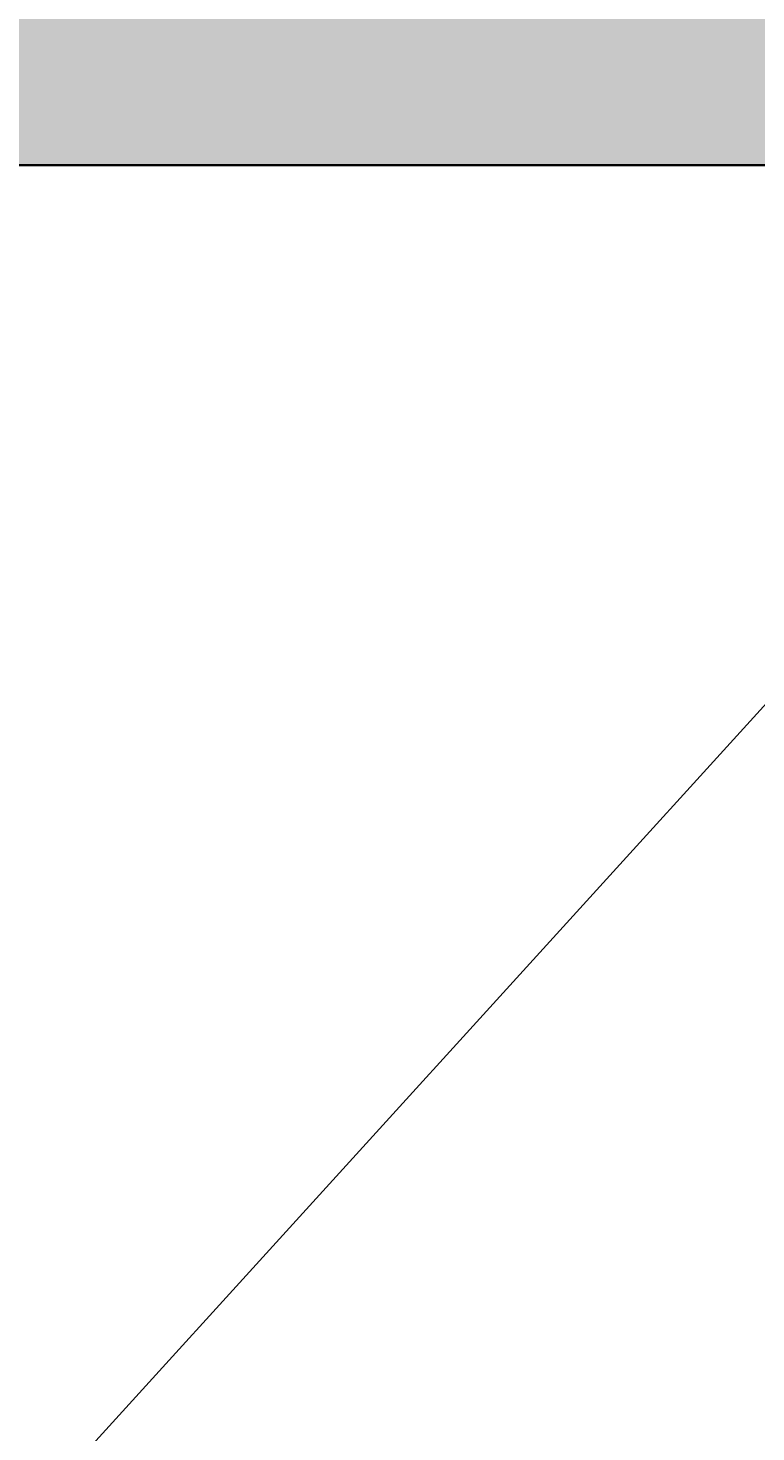
# Model space of a CAD drawing. Units: inches. Extents: x 1998 to 2588, y 1139 to 1977.
# Tile 37 of 134: x 2257 to 2275, y 1557 to 1592. Entities that reach past the tile are written whole.
import ezdxf

# ---------------------------------------------------------------- set-up
doc = ezdxf.new("R2010")
doc.units = ezdxf.units.IN
for name, color, linetype, lineweight in [('A-ANNO-DIMS', 2, 'Continuous', 18), ('A-FLOR-OPEN', 8, 'Continuous', 18), ('A-WALL-PATT', 252, 'Continuous', 13), ('WALL', 200, 'Continuous', 35)]:
    doc.layers.add(name, color=color, linetype=linetype, lineweight=lineweight)
doc.styles.get("Standard").update_dxf_attribs({"font": 'arial.ttf'})
doc.dimstyles.get("Standard").update_dxf_attribs({"dimtxt": 0.18, "dimasz": 0.18, "dimexe": 0.18, "dimexo": 0.0625, "dimgap": 0.09, "dimtad": 0, "dimtih": 1, "dimtoh": 1, "dimdec": 4, "dimzin": 0, "dimdsep": 46, "dimtxsty": 'Standard', "dimcen": 0.09, "dimadec": 0, "dimazin": 0, "dimtfac": 1, "dimtdec": 4, "dimtofl": 0, "dimtmove": 0, "dimatfit": 3, "dimfxl": 1, "dimtolj": 1, "dimtzin": 0, "dimarcsym": 0})

# ---------------------------------------------------------------- blocks, each defined once
blk = doc.blocks.new('*D34')
at = {"layer": 'A-ANNO-DIMS', "color": 0, "lineweight": -2, "transparency": 16777216}
for p, q in [((2407.91, 1594.732), (1997.843, 1594.732)), ((1998.023, 1594.552), (1998.023, 1558.913)), ((1998.023, 1522.912), (1998.023, 1558.552)), ((2407.91, 1522.732), (1997.843, 1522.732))]:
    blk.add_line(p, q, dxfattribs=at)
at = {"layer": 'A-ANNO-DIMS', "color": 0, "transparency": 16777216}
for points in [[(1997.993, 1594.552), (1998.053, 1594.552), (1998.023, 1594.732)], [(1997.993, 1522.912), (1998.053, 1522.912), (1998.023, 1522.732)]]:
    blk.add_solid(points, dxfattribs=at)
at = {"layer": 'Defpoints', "color": 0, "transparency": 16777216}
for p in [(1998.023, 1594.732), (2407.973, 1594.732), (2407.973, 1522.732)]:
    blk.add_point(p, dxfattribs=at)
at = {"layer": 'A-ANNO-DIMS', "color": 0, "transparency": 16777216, "insert": (1998.023, 1558.732), "char_height": 0.18, "attachment_point": 5}
blk.add_mtext('\\A1;72', dxfattribs=at)
blk = doc.blocks.new('*D41')
at = {"layer": 'A-ANNO-DIMS', "color": 0, "lineweight": -2, "transparency": 16777216}
for p, q in [((2227.473, 1588.67), (2227.473, 1138.602)), ((2287.473, 1588.67), (2287.473, 1138.602)), ((2227.653, 1138.782), (2257.254, 1138.782)), ((2287.293, 1138.782), (2257.692, 1138.782))]:
    blk.add_line(p, q, dxfattribs=at)
at = {"layer": 'A-ANNO-DIMS', "color": 0, "transparency": 16777216}
for points in [[(2227.653, 1138.812), (2227.653, 1138.752), (2227.473, 1138.782)], [(2287.293, 1138.812), (2287.293, 1138.752), (2287.473, 1138.782)]]:
    blk.add_solid(points, dxfattribs=at)
at = {"layer": 'Defpoints', "color": 0, "transparency": 16777216}
for p in [(2227.473, 1588.732), (2287.473, 1588.732), (2287.473, 1138.782)]:
    blk.add_point(p, dxfattribs=at)
at = {"layer": 'A-ANNO-DIMS', "color": 0, "transparency": 16777216, "insert": (2257.473, 1138.782), "char_height": 0.18, "attachment_point": 5}
blk.add_mtext('\\A1;60', dxfattribs=at)

msp = doc.modelspace()

# ---------------------------------------------------------------- hatches: boundary and pattern name
at = {"layer": 'A-WALL-PATT'}
h = msp.add_hatch(color=256, dxfattribs=at)
h.dxf.hatch_style = 1
h.paths.add_polyline_path([(2222.9729, 1888.7324), (2099.4125, 1888.7324), (2099.4125, 1879.7324), (2222.9729, 1879.7324)])
h.paths.add_polyline_path([(2096.9729, 1868.3278), (2087.9729, 1868.3278), (2087.9729, 1775.637), (2096.9729, 1775.637)])
h.paths.add_polyline_path([(2227.4729, 1868.3278), (2222.9729, 1868.3278), (2222.9729, 1774.3318), (2227.4729, 1774.3318)])
h.paths.add_polyline_path([(2188.3019, 1759.7324), (2138.6074, 1759.7324), (2099.4125, 1759.7324), (2099.4125, 1755.2324), (2176.9729, 1755.2324), (2188.3019, 1755.2324)])
h.paths.add_polyline_path([(2087.9729, 1759.7324), (2059.4729, 1759.7324), (2059.4729, 1702.7324), (2087.9729, 1702.7324), (2087.9729, 1707.2324), (2063.9729, 1707.2324), (2063.9729, 1755.2324), (2087.9729, 1755.2324)])
h.paths.add_polyline_path([(2096.9729, 1755.2324), (2087.9729, 1755.2324), (2087.9729, 1707.2324), (2096.9729, 1707.2324)])
h.paths.add_polyline_path([(2187.0461, 1707.2324), (2105.9729, 1707.2324), (2096.9729, 1707.2324), (2087.9729, 1707.2324), (2087.9729, 1702.7324), (2105.9729, 1702.7324), (2114.9729, 1702.7324), (2187.0461, 1702.7324)])
h.paths.add_polyline_path([(2181.4729, 1719.2028), (2176.9729, 1719.2028), (2176.9729, 1707.2324), (2181.4729, 1707.2324)])
h.paths.add_polyline_path([(2216.0332, 1588.7324), (2114.9729, 1588.7324), (2105.9729, 1588.7324), (2105.9729, 1584.2324), (2216.0332, 1584.2324)])
h.paths.add_polyline_path([(2077.691, 1588.7324), (2061.4729, 1588.7324), (2061.4729, 1584.2324), (2077.691, 1584.2324)])
h.paths.add_polyline_path([(2105.9729, 1588.7324), (2098.0956, 1588.7324), (2098.0956, 1584.2324), (2105.9729, 1584.2324)])
h.paths.add_polyline_path([(2114.9729, 1596.2642), (2110.1012, 1596.2642), (2105.9729, 1596.2642), (2105.9729, 1588.7324), (2114.9729, 1588.7324)])
h.paths.add_polyline_path([(2114.9729, 1584.2324), (2105.9729, 1584.2324), (2105.9729, 1580.249), (2110.1012, 1580.249), (2114.9729, 1580.249)])
h.paths.add_polyline_path([(2114.9729, 1547.7716), (2110.1012, 1547.7716, -0.0318759), (2105.9729, 1548.035), (2105.9729, 1470.2324), (2108.3775, 1470.2324), (2108.3775, 1465.7324), (2186.2943, 1465.7324), (2186.2943, 1470.2324), (2114.9729, 1470.2324)])
h.paths.add_polyline_path([(2227.4729, 1584.2324), (2222.9729, 1584.2324), (2222.9729, 1486.137), (2227.4729, 1486.137)])
h.paths.add_polyline_path([(2295.4138, 1593.2324), (2227.4729, 1593.2324), (2227.4729, 1588.7324), (2295.4138, 1588.7324), (2295.4138, 1591.8729)])
h.paths.add_polyline_path([(2345.9729, 1627.1165), (2341.4729, 1627.1165), (2341.4729, 1593.2324), (2337.2869, 1593.2324), (2337.2869, 1591.8729), (2337.2869, 1588.7324), (2345.9729, 1588.7324)])
h.paths.add_polyline_path([(2291.9729, 1588.7324), (2287.4729, 1588.7324), (2287.4729, 1522.7324), (2291.9729, 1522.7324)])
h.paths.add_polyline_path([(2291.9729, 1522.7324), (2287.4729, 1522.7324), (2227.4729, 1522.7324), (2227.4729, 1518.2324), (2291.9729, 1518.2324)])
h.paths.add_polyline_path([(2295.7347, 1519.5919), (2295.7347, 1522.7324), (2291.9729, 1522.7324), (2291.9729, 1518.2324), (2295.7347, 1518.2324)])
h.paths.add_polyline_path([(2345.9729, 1522.7324), (2337.6078, 1522.7324), (2337.6078, 1519.5919), (2337.6078, 1518.2324), (2341.4729, 1518.2324), (2341.4729, 1488.5616), (2345.9729, 1488.5616)])
h.paths.add_polyline_path([(2345.9729, 1468.1569), (2341.4729, 1468.1569), (2341.4729, 1374.2324), (2227.4729, 1374.2324), (2227.4729, 1369.7324), (2345.9729, 1369.7324)])
h.paths.add_polyline_path([(2345.9729, 1369.7324), (2341.4729, 1369.7324), (2341.4729, 1362.2324), (2345.9729, 1362.2324)])
h.paths.add_polyline_path([(2345.9729, 1317.7324), (2345.9729, 1322.2324), (2341.4729, 1322.2324), (2341.4729, 1285.137), (2345.9729, 1285.137)], flags=17)
h.paths.add_polyline_path([(2356.2096, 1322.2324), (2345.9729, 1322.2324), (2345.9729, 1317.7324), (2356.2096, 1317.7324), (2356.2096, 1319.3088)], flags=17)
h.paths.add_polyline_path([(2393.9729, 1322.2324), (2375.6999, 1322.2324), (2375.6999, 1319.3088, -0.0202458), (2375.636, 1317.7324), (2393.9729, 1317.7324)], flags=17)
h.paths.add_polyline_path([(2398.4729, 1322.2324), (2393.9729, 1322.2324), (2393.9729, 1317.7324), (2393.9729, 1237.7324), (2345.9729, 1237.7324), (2345.9729, 1264.7324), (2341.4729, 1264.7324), (2341.4729, 1228.7324), (2393.9729, 1228.7324), (2482.7412, 1228.7324), (2482.7412, 1237.7324), (2398.4729, 1237.7324), (2398.4729, 1297.1029)])
h.paths.add_polyline_path([(2398.4729, 1362.2324), (2393.9729, 1362.2324), (2393.9729, 1357.7324), (2398.4729, 1357.7324)])
h.paths.add_polyline_path([(2345.9729, 1329.7549), (2341.4729, 1329.7549), (2341.4729, 1322.2324), (2345.9729, 1322.2324)])

# ---------------------------------------------------------------- linework, layer by layer
at = {"layer": 'A-FLOR-OPEN'}
msp.add_line((2227.4729, 1522.7324), (2287.4729, 1588.7324), dxfattribs=at)
at = {"layer": 'WALL'}
msp.add_line((2295.4138, 1588.7324), (2227.4729, 1588.7324), dxfattribs=at)

# ---------------------------------------------------------------- dimensions: what is measured, and where the dimension line sits
at = {"layer": 'A-ANNO-DIMS'}
dim = msp.add_linear_dim(base=(1998.0229, 1594.7324), p1=(2407.9729, 1522.7324), p2=(2407.9729, 1594.7324), angle=90, dimstyle='Standard', override={"dimdec": 0, "dimlfac": 1, "dimrnd": 0, "dimzin": 0, "dimdsep": 46, "dimlunit": 2}, dxfattribs=at)
dim.commit()
dim.dimension.update_dxf_attribs({"geometry": '*D34', "text_midpoint": (1998.0229, 1558.7324)})
dim = msp.add_linear_dim(base=(2287.4729, 1138.7824), p1=(2227.4729, 1588.7324), p2=(2287.4729, 1588.7324), dimstyle='Standard', override={"dimdec": 0, "dimlfac": 1, "dimrnd": 0, "dimzin": 0, "dimdsep": 46, "dimlunit": 2}, dxfattribs=at)
dim.commit()
dim.dimension.update_dxf_attribs({"geometry": '*D41', "text_midpoint": (2257.4729, 1138.7824)})

doc.saveas('drawing.dxf')
